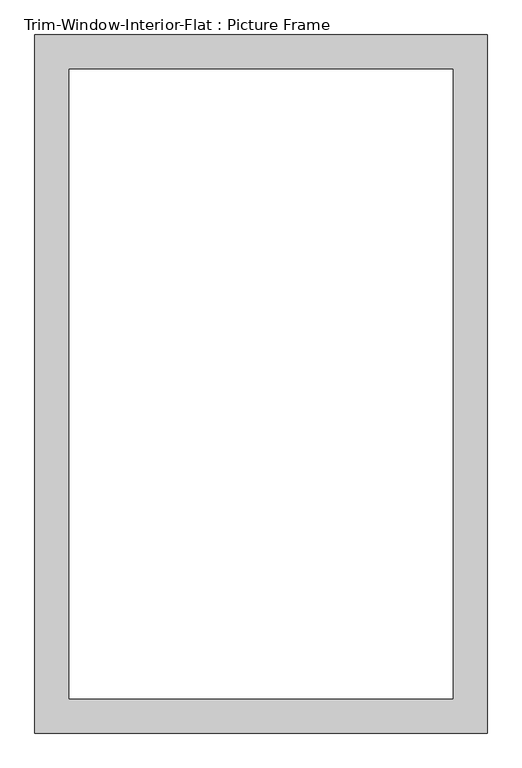
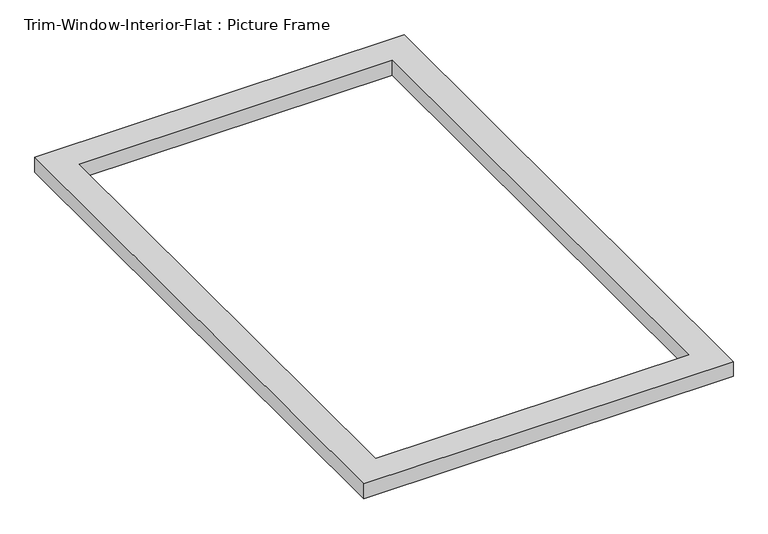
"""IFC4 building model written with IfcOpenShell, lengths in millimetres: proxy geometry, Trim-Window-Interior-Flat : Picture Frame."""

from ifc_helpers import new_model, si_unit, origin, origin_with_axes, place, context, project, spatial, polyline, outline, extrude, source, transform, mapped, element, save


def trim_window_interior_flat_picture_frame_80babb00(model_context):
    return source(origin(), model_context, "Body", "SweptSolid", [
        extrude(outline(polyline([(374.65, -44.45), (-374.65, -44.45), (-374.65, 1111.25), (374.65, 1111.25), (374.65, -44.45)]), holes=[polyline([(317.5, 12.7), (317.5, 1054.1), (-317.5, 1054.1), (-317.5, 12.7), (317.5, 12.7)])]), origin_with_axes(), (0.0, 0.0, 1.0), 31.75),
    ])


if __name__ == "__main__":
    model = new_model("IFC4")
    model_context = context("Model", 3, world=origin())
    ifc_project = project(units=[si_unit("LENGTHUNIT", "METRE", prefix="MILLI")], contexts=[model_context])
    site = spatial("IfcSite", under=ifc_project)
    building = spatial("IfcBuilding", under=site)
    placement = place(None, origin())
    trim_window_interior_flat_picture_frame_shape = trim_window_interior_flat_picture_frame_80babb00(model_context)
    element("IfcBuildingElementProxy", 1, Name="Trim-Window-Interior-Flat : Picture Frame", ObjectType="Trim-Window-Interior-Flat : Picture Frame", at=placement, inside=building, context=model_context, shape_type="MappedRepresentation", body=[
        mapped(trim_window_interior_flat_picture_frame_shape, transform((0.0, 0.0, 0.0), x_axis=(1.0, 0.0, 0.0), y_axis=(0.0, 1.0, 0.0), z_axis=(0.0, 0.0, 1.0))),
    ])
    save(model, "model.ifc")

# Revit data of these elements
# Type "Trim-Window-Interior-Flat : Picture Frame"
#   Trim Thickness_Picture Frame = 0' - 1 1/4"
#   Trim Width = 0' - 2 1/4"
#   Trim Thickness_with Sill = 0' - 0 3/4"
#   Sill Thickness = 0' - 1 1/4"
#   Opening Width [instance default] = 2' - 0"
#   Opening Height [instance default] = 3' - 0"
#   Default Elevation = 4' - 0"
#   Sill = no
#   Picture Frame = yes
#   Trim Material [instance default] = none
# Element 1 (IfcBuildingElementProxy, "Trim-Window-Interior-Flat : Picture Frame")
#   Opening Width = 2' - 2"
#   Opening Height = 3' - 6"
#   Trim Material = Wood - Stained
#   Materials on its faces: "Wood - Stained"
# Materials
#   "Wood - Stained": class "Wood", colour RGB 224 178 126, transparency 0, Cost = 0
